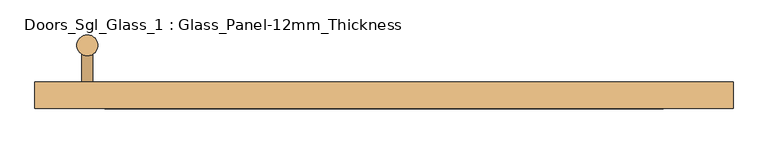
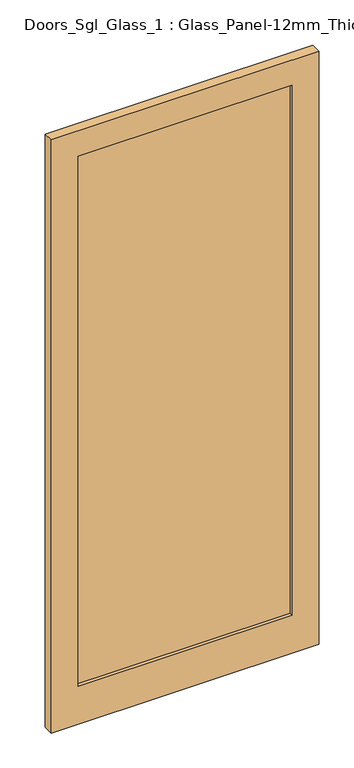
"""IFC4 building model written with IfcOpenShell, lengths in millimetres: door geometry, Doors_Sgl_Glass_1 : Glass_Panel-12mm_Thickness."""

from ifc_helpers import new_model, si_unit, point, frame, frame_2d, origin, place, context, project, spatial, polyline, circle_curve, trimmed, segment, composite_curve, outline, extrude, source, transform, mapped, element, save


def doors_sgl_glass_1_glass_panel_12mm_thickness_6ba6481b(model_context):
    return source(origin(), model_context, "Body", "SweptSolid", [
        extrude(outline(polyline([(399.7400148, 50.0), (399.7400148, 38.0), (-399.7400148, 38.0), (-399.7400148, 50.0), (399.7400148, 50.0)])), frame((0.0, 0.0, 150.0), z_axis=(0.0, 0.0, 1.0), x_axis=(1.0, 0.0, 0.0)), (0.0, 0.0, 1.0), 2090.0242188),
        extrude(outline(polyline([(0.0, -499.7400148), (0.0, 499.7400148), (2340.0242188, 499.7400148), (2340.0242188, -499.7400148), (0.0, -499.7400148)]), holes=[polyline([(2240.0242188, 399.7400148), (150.0, 399.7400148), (150.0, -399.7400148), (2240.0242188, -399.7400148), (2240.0242188, 399.7400148)])]), frame((0.0, 25.0, 0.0), z_axis=(0.0, 1.0, 0.0), x_axis=(0.0, 0.0, 1.0)), (0.0, 0.0, 1.0), 38.0),
        extrude(outline(composite_curve([segment(trimmed(circle_curve(frame_2d((1450.0, -424.7400148)), 8.0), [point((1450.0, -416.7400148))], [point((1450.0, -432.7400148))], False, "CARTESIAN"), True, "CONTINUOUS"), segment(trimmed(circle_curve(frame_2d((1450.0, -424.7400148)), 8.0), [point((1450.0, -432.7400148))], [point((1450.0, -416.7400148))], False, "CARTESIAN"), True, "CONTINUOUS")], self_intersect=False)), frame((0.0, 63.0, 0.0), z_axis=(0.0, 1.0, 0.0), x_axis=(0.0, 0.0, 1.0)), (0.0, 0.0, 1.0), 53.0),
        extrude(outline(composite_curve([segment(trimmed(circle_curve(frame_2d((750.0, -424.7400148)), 8.0), [point((750.0, -416.7400148))], [point((750.0, -432.7400148))], False, "CARTESIAN"), True, "CONTINUOUS"), segment(trimmed(circle_curve(frame_2d((750.0, -424.7400148)), 8.0), [point((750.0, -432.7400148))], [point((750.0, -416.7400148))], False, "CARTESIAN"), True, "CONTINUOUS")], self_intersect=False)), frame((0.0, 63.0, 0.0), z_axis=(0.0, 1.0, 0.0), x_axis=(0.0, 0.0, 1.0)), (0.0, 0.0, 1.0), 53.0),
        extrude(outline(composite_curve([segment(trimmed(circle_curve(frame_2d((-424.7400148, 116.0)), 15.0), [point((-424.7400148, 101.0))], [point((-424.7400148, 131.0))], False, "CARTESIAN"), True, "CONTINUOUS"), segment(trimmed(circle_curve(frame_2d((-424.7400148, 116.0)), 15.0), [point((-424.7400148, 131.0))], [point((-424.7400148, 101.0))], False, "CARTESIAN"), True, "CONTINUOUS")], self_intersect=False)), frame((0.0, 0.0, 650.0), z_axis=(0.0, 0.0, 1.0), x_axis=(1.0, 0.0, 0.0)), (0.0, 0.0, 1.0), 900.0),
    ])


if __name__ == "__main__":
    model = new_model("IFC4")
    model_context = context("Model", 3, world=origin())
    ifc_project = project(units=[si_unit("LENGTHUNIT", "METRE", prefix="MILLI")], contexts=[model_context])
    site = spatial("IfcSite", under=ifc_project)
    building = spatial("IfcBuilding", under=site)
    placement = place(None, origin())
    doors_sgl_glass_1_glass_panel_12mm_thickness_shape = doors_sgl_glass_1_glass_panel_12mm_thickness_6ba6481b(model_context)
    element("IfcDoor", 1, ObjectType="Doors_Sgl_Glass_1 : Glass_Panel-12mm_Thickness", at=placement, inside=building, context=model_context, shape_type="MappedRepresentation", body=[
        mapped(doors_sgl_glass_1_glass_panel_12mm_thickness_shape, transform((0.0, 0.0, 0.0), x_axis=(1.0, 0.0, 0.0), y_axis=(0.0, 1.0, 0.0), z_axis=(0.0, 0.0, 1.0))),
    ])
    save(model, "model.ifc")

# Revit data of these elements
# Type "Doors_Sgl_Glass_1 : Glass_Panel-12mm_Thickness"
#   Type Mark = "60"
#   Construction Type Id = "GSP4R"
#   Keynote = "H11"
#   Analytic Construction = "1/8 in Pilkington single glazing"
#   Visual Light Transmittance = 0.9
#   Stile Top Rail = 0' - 3.93701"
#   Stile Shutting = 0' - 3.93701"
#   Stile Hanging = 0' - 3.93701"
#   Stile Bottom Rail = 0' - 5.90551"
#   Solar Heat Gain Coefficient = 0.78
#   Offset = 0' - 1.9685"
#   Heat Transfer Coefficient (U) = 3.6886 W/(m²·K)
#   Handle X Distance = 0' - 2.95276"
#   Glazing Thickness = 0' - 0.47244"
#   Define Thermal Properties by = 1
#   Material Ironmongery = Metal - Aluminum
#   Material Frame = Metal - Aluminum
#   Material Glass = Glass
#   Function = (empty or 0)
# Element 1 (IfcDoor, "Doors_Sgl_Glass_1 : Glass_Panel-12mm_Thickness")
#   Materials on its faces: "Metal - Aluminum", "Glass"
# Materials
#   "Metal - Aluminum": class "Metal", colour RGB 247 247 247, transparency 0
#   "Glass": class "Glass", colour RGB 0 128 192, transparency 0.9, Description = "Soda Lime Glass", Cost = 0
